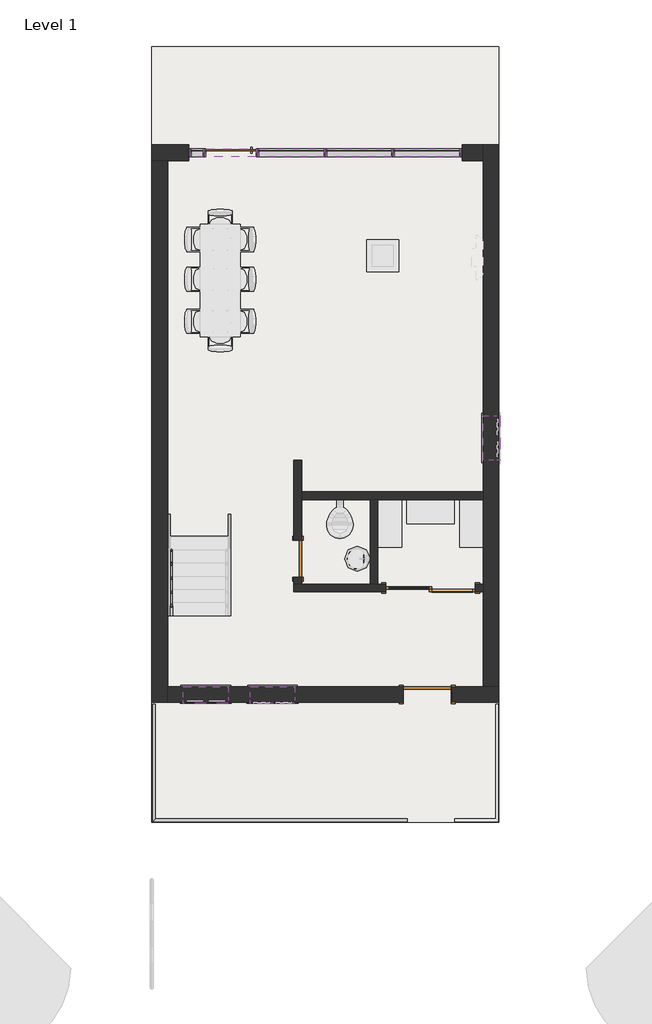
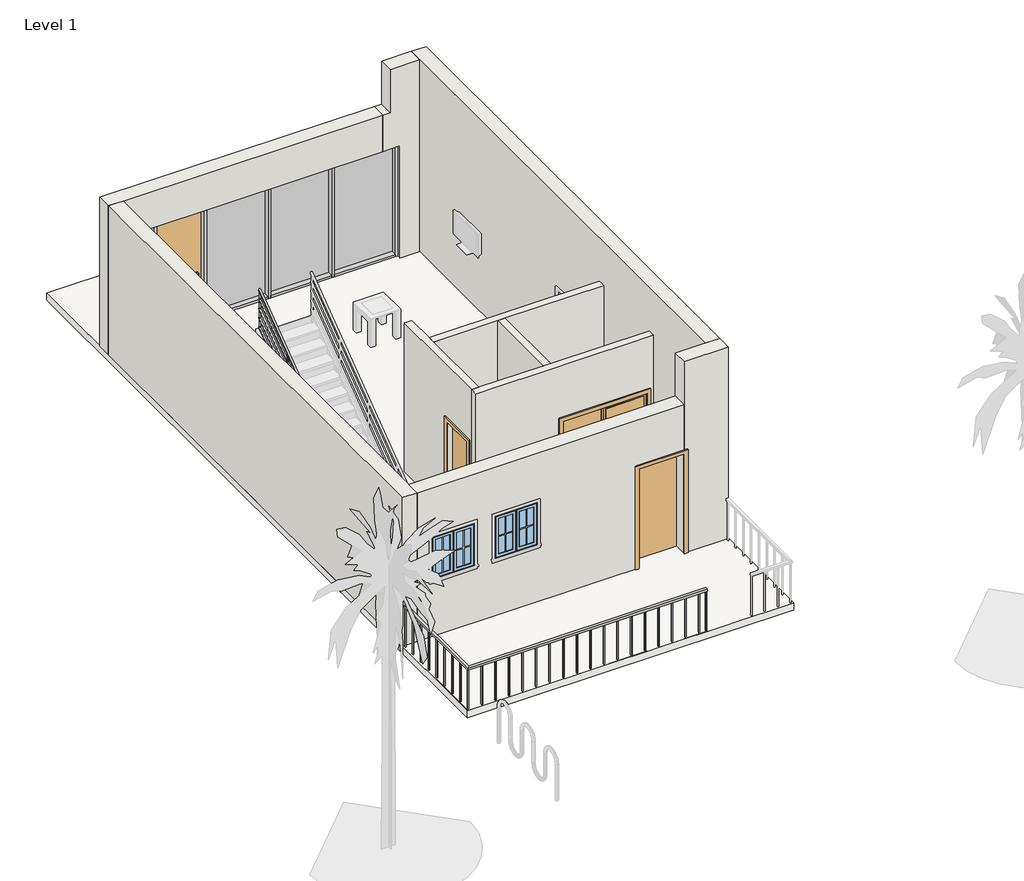
# One storey, part 1 of 2: 15 members, 10 walls, 4 doors, 4 plates, 3 windows, 2 railings, 1 slab.
"""IFC4 building model written with IfcOpenShell, lengths in millimetres."""

from ifc_helpers import new_model, si_unit, frame, origin, origin_with_axes, place, context, project, spatial, polyline, circle_curve, ellipse_curve, outline, extrude, faceted_brep, transform, mapped, element, save
from ifc_brep_helpers import plane_surface, cylinder_surface, advanced_brep
from components import m_door_curtain_wall_single_glass_m_door_curtain_wall_single_92f462ab, m_door_double_sliding_1700_x_2000mm_d36f6dca, m_single_flush_0915_x_2134mm_9cebaac8, m_single_flush_700x1980_d4223ffa, rectangular_mullion_50_x_150mm_6225e4e3, rectangular_mullion_50_x_150mm_662c37b1, rectangular_mullion_50_x_150mm_ef1c4831, rectangular_mullion_50_x_150mm_c6e312d8, rectangular_mullion_50_x_150mm_a74c1b10, rectangular_mullion_50_x_150mm_bd48bb75, system_panel_glazed_6a0df73a, system_panel_glazed_b955046d, m_window_casement_double_850_x_900mm_d87c3818, m_window_casement_double_850_x_900mm_ced1a82e

model = new_model("IFC4")

# Units and contexts
model_context = context("Model", 3, world=origin())
ifc_project = project(units=[si_unit("LENGTHUNIT", "METRE", prefix="MILLI")], contexts=[model_context])

# Site, building, storey
site = spatial("IfcSite", under=ifc_project)
building = spatial("IfcBuilding", under=site)
storey = spatial("IfcBuildingStorey", under=building, Name="Level 1", Elevation=0.0)

# Doors
placement = place(None, origin())
m_door_curtain_wall_single_glass_m_door_curtain_wall_single_shape = m_door_curtain_wall_single_glass_m_door_curtain_wall_single_92f462ab(model_context)
element("IfcDoor", 1, ObjectType="M_Door-Curtain-Wall-Single-Glass : M_Door-Curtain-Wall-Single-Glass", at=placement, inside=storey, context=model_context, shape_type="MappedRepresentation", body=[
    mapped(m_door_curtain_wall_single_glass_m_door_curtain_wall_single_shape, transform((-3862.7817551, 6033.2522499, 0.0), x_axis=(-1.0, 0.0, 0.0), y_axis=(0.0, -1.0, 0.0), z_axis=(0.0, 0.0, 1.0))),
])
m_door_double_sliding_1700_x_2000mm_shape = m_door_double_sliding_1700_x_2000mm_d36f6dca(model_context)
element("IfcDoor", 2, ObjectType="M_Door-Double-Sliding : 1700 x 2000mm", at=placement, inside=storey, context=model_context, shape_type="MappedRepresentation", body=[
    mapped(m_door_double_sliding_1700_x_2000mm_shape, transform((-69.0317552, -2114.7477501, 0.0), x_axis=(-1.0, 0.0, 0.0), y_axis=(0.0, -1.0, 0.0), z_axis=(0.0, 0.0, 1.0))),
])
m_single_flush_0915_x_2134mm_shape = m_single_flush_0915_x_2134mm_9cebaac8(model_context)
element("IfcDoor", 3, ObjectType="M_Single-Flush : 0915 x 2134mm", at=placement, inside=storey, context=model_context, shape_type="MappedRepresentation", body=[
    mapped(m_single_flush_0915_x_2134mm_shape, transform((-131.5317552, -4266.7477501, 0.0), x_axis=(1.0, 0.0, 0.0), y_axis=(0.0, 1.0, 0.0), z_axis=(0.0, 0.0, 1.0))),
])
m_single_flush_700x1980_shape = m_single_flush_700x1980_d4223ffa(model_context)
element("IfcDoor", 4, ObjectType="M_Single-Flush : 700x1980", at=placement, inside=storey, context=model_context, shape_type="MappedRepresentation", body=[
    mapped(m_single_flush_700x1980_shape, transform((-2594.0317552, -1685.7477501, 0.0), x_axis=(0.0, -1.0, 0.0), y_axis=(1.0, 0.0, 0.0), z_axis=(0.0, 0.0, 1.0))),
])

# Members
rectangular_mullion_50_x_150mm_shape = rectangular_mullion_50_x_150mm_6225e4e3(model_context)
element("IfcMember", 5, ObjectType="Rectangular Mullion : 50 x 150mm", at=placement, inside=storey, context=model_context, shape_type="MappedRepresentation", body=[
    mapped(rectangular_mullion_50_x_150mm_shape, transform((-3356.531755, 6033.2522499, 0.0), x_axis=(1.0, 0.0, 0.0), y_axis=(0.0, -1.0, 0.0), z_axis=(0.0, 0.0, -1.0))),
])
element("IfcMember", 6, ObjectType="Rectangular Mullion : 50 x 150mm", at=placement, inside=storey, context=model_context, shape_type="MappedRepresentation", body=[
    mapped(rectangular_mullion_50_x_150mm_shape, transform((-2069.0317552, 6033.2522499, 0.0), x_axis=(1.0, 0.0, 0.0), y_axis=(0.0, -1.0, 0.0), z_axis=(0.0, 0.0, -1.0))),
])
element("IfcMember", 7, ObjectType="Rectangular Mullion : 50 x 150mm", at=placement, inside=storey, context=model_context, shape_type="MappedRepresentation", body=[
    mapped(rectangular_mullion_50_x_150mm_shape, transform((-781.5317553, 6033.2522499, 0.0), x_axis=(1.0, 0.0, 0.0), y_axis=(0.0, -1.0, 0.0), z_axis=(0.0, 0.0, -1.0))),
])
element("IfcMember", 8, ObjectType="Rectangular Mullion : 50 x 150mm", at=placement, inside=storey, context=model_context, shape_type="MappedRepresentation", body=[
    mapped(rectangular_mullion_50_x_150mm_shape, transform((-4369.0317552, 6033.2522499, 0.0), x_axis=(1.0, 0.0, 0.0), y_axis=(0.0, -1.0, 0.0), z_axis=(0.0, 0.0, -1.0))),
])
rectangular_mullion_50_x_150mm_2_shape = rectangular_mullion_50_x_150mm_662c37b1(model_context)
element("IfcMember", 9, ObjectType="Rectangular Mullion : 50 x 150mm", at=placement, inside=storey, context=model_context, shape_type="MappedRepresentation", body=[
    mapped(rectangular_mullion_50_x_150mm_2_shape, transform((530.9682448, 6033.2522499, 0.0), x_axis=(1.0, 0.0, 0.0), y_axis=(0.0, -1.0, 0.0), z_axis=(0.0, 0.0, -1.0))),
])
element("IfcMember", 10, ObjectType="Rectangular Mullion : 50 x 150mm", at=placement, inside=storey, context=model_context, shape_type="MappedRepresentation", body=[
    mapped(rectangular_mullion_50_x_150mm_2_shape, transform((-4669.0317552, 6033.2522499, 2400.0), x_axis=(-1.0, 0.0, 0.0), y_axis=(0.0, -1.0, 0.0), z_axis=(0.0, 0.0, 1.0))),
])
rectangular_mullion_50_x_150mm_3_shape = rectangular_mullion_50_x_150mm_ef1c4831(model_context)
element("IfcMember", 11, ObjectType="Rectangular Mullion : 50 x 150mm", at=placement, inside=storey, context=model_context, shape_type="MappedRepresentation", body=[
    mapped(rectangular_mullion_50_x_150mm_3_shape, transform((-4619.0317552, 6033.2522499, 0.0), x_axis=(0.0, 0.0, -1.0), y_axis=(0.0, -1.0, 0.0), z_axis=(-1.0, 0.0, 0.0))),
])
element("IfcMember", 12, ObjectType="Rectangular Mullion : 50 x 150mm", at=placement, inside=storey, context=model_context, shape_type="MappedRepresentation", body=[
    mapped(rectangular_mullion_50_x_150mm_3_shape, transform((-4394.0317552, 6033.2522499, 2400.0), x_axis=(0.0, 0.0, 1.0), y_axis=(0.0, -1.0, 0.0), z_axis=(1.0, 0.0, 0.0))),
])
rectangular_mullion_50_x_150mm_4_shape = rectangular_mullion_50_x_150mm_c6e312d8(model_context)
element("IfcMember", 13, ObjectType="Rectangular Mullion : 50 x 150mm", at=placement, inside=storey, context=model_context, shape_type="MappedRepresentation", body=[
    mapped(rectangular_mullion_50_x_150mm_4_shape, transform((480.9682448, 6033.2522499, 2400.0), x_axis=(0.0, 0.0, 1.0), y_axis=(0.0, -1.0, 0.0), z_axis=(1.0, 0.0, 0.0))),
])
element("IfcMember", 14, ObjectType="Rectangular Mullion : 50 x 150mm", at=placement, inside=storey, context=model_context, shape_type="MappedRepresentation", body=[
    mapped(rectangular_mullion_50_x_150mm_4_shape, transform((-2094.0317552, 6033.2522499, 2400.0), x_axis=(0.0, 0.0, 1.0), y_axis=(0.0, -1.0, 0.0), z_axis=(1.0, 0.0, 0.0))),
])
element("IfcMember", 15, ObjectType="Rectangular Mullion : 50 x 150mm", at=placement, inside=storey, context=model_context, shape_type="MappedRepresentation", body=[
    mapped(rectangular_mullion_50_x_150mm_4_shape, transform((-806.5317553, 6033.2522499, 2400.0), x_axis=(0.0, 0.0, 1.0), y_axis=(0.0, -1.0, 0.0), z_axis=(1.0, 0.0, 0.0))),
])
rectangular_mullion_50_x_150mm_5_shape = rectangular_mullion_50_x_150mm_a74c1b10(model_context)
element("IfcMember", 16, ObjectType="Rectangular Mullion : 50 x 150mm", at=placement, inside=storey, context=model_context, shape_type="MappedRepresentation", body=[
    mapped(rectangular_mullion_50_x_150mm_5_shape, transform((-3381.531755, 6033.2522499, 2400.0), x_axis=(0.0, 0.0, 1.0), y_axis=(0.0, -1.0, 0.0), z_axis=(1.0, 0.0, 0.0))),
])
rectangular_mullion_50_x_150mm_6_shape = rectangular_mullion_50_x_150mm_bd48bb75(model_context)
element("IfcMember", 17, ObjectType="Rectangular Mullion : 50 x 150mm", at=placement, inside=storey, context=model_context, shape_type="MappedRepresentation", body=[
    mapped(rectangular_mullion_50_x_150mm_6_shape, transform((-3331.531755, 6033.2522499, 0.0), x_axis=(0.0, 0.0, -1.0), y_axis=(0.0, -1.0, 0.0), z_axis=(-1.0, 0.0, 0.0))),
])
element("IfcMember", 18, ObjectType="Rectangular Mullion : 50 x 150mm", at=placement, inside=storey, context=model_context, shape_type="MappedRepresentation", body=[
    mapped(rectangular_mullion_50_x_150mm_6_shape, transform((-2044.0317552, 6033.2522499, 0.0), x_axis=(0.0, 0.0, -1.0), y_axis=(0.0, -1.0, 0.0), z_axis=(-1.0, 0.0, 0.0))),
])
element("IfcMember", 19, ObjectType="Rectangular Mullion : 50 x 150mm", at=placement, inside=storey, context=model_context, shape_type="MappedRepresentation", body=[
    mapped(rectangular_mullion_50_x_150mm_6_shape, transform((-756.5317553, 6033.2522499, 0.0), x_axis=(0.0, 0.0, -1.0), y_axis=(0.0, -1.0, 0.0), z_axis=(-1.0, 0.0, 0.0))),
])

# Plates
system_panel_glazed_shape = system_panel_glazed_6a0df73a(model_context)
element("IfcPlate", 20, ObjectType="System Panel : Glazed", at=placement, inside=storey, context=model_context, shape_type="MappedRepresentation", body=[
    mapped(system_panel_glazed_shape, transform((-4506.5317552, 6033.2522499, 50.0), x_axis=(1.0, 0.0, 0.0), y_axis=(0.0, 1.0, 0.0), z_axis=(0.0, 0.0, 1.0))),
])
system_panel_glazed_2_shape = system_panel_glazed_b955046d(model_context)
element("IfcPlate", 21, ObjectType="System Panel : Glazed", at=placement, inside=storey, context=model_context, shape_type="MappedRepresentation", body=[
    mapped(system_panel_glazed_2_shape, transform((-137.7817553, 6033.2522499, 50.0), x_axis=(1.0, 0.0, 0.0), y_axis=(0.0, 1.0, 0.0), z_axis=(0.0, 0.0, 1.0))),
])
element("IfcPlate", 22, ObjectType="System Panel : Glazed", at=placement, inside=storey, context=model_context, shape_type="MappedRepresentation", body=[
    mapped(system_panel_glazed_2_shape, transform((-1425.2817553, 6033.2522499, 50.0), x_axis=(1.0, 0.0, 0.0), y_axis=(0.0, 1.0, 0.0), z_axis=(0.0, 0.0, 1.0))),
])
element("IfcPlate", 23, ObjectType="System Panel : Glazed", at=placement, inside=storey, context=model_context, shape_type="MappedRepresentation", body=[
    mapped(system_panel_glazed_2_shape, transform((-2712.7817551, 6033.2522499, 50.0), x_axis=(1.0, 0.0, 0.0), y_axis=(0.0, 1.0, 0.0), z_axis=(0.0, 0.0, 1.0))),
])

# Railings
element("IfcRailing", 24, ObjectType="900mm Pipe", at=placement, inside=storey, context=model_context, shape_type="AdvancedBrep", body=[
    advanced_brep(
    [(-4973.6317552, -2766.7477501, 1063.1999558), (-5013.6317552, -2766.7477501, 1063.1999558), (-4973.6317552, 1233.2522499, 4074.9646617), (-5013.6317552, 1233.2522499, 4074.9646617)],
    [
        (0, 1, ellipse_curve(frame((-4993.6317552, -2766.7477501, 1063.1999558), z_axis=(0.0, -1.0, 0.0), x_axis=(0.0, 0.0, -1.0)), 25.0353383, 20.0)),
        (1, 0, ellipse_curve(frame((-4993.6317552, -2766.7477501, 1063.1999558), z_axis=(0.0, -1.0, 0.0), x_axis=(0.0, 0.0, -1.0)), 25.0353383, 20.0)),
        (2, 3, ellipse_curve(frame((-4993.6317552, 1233.2522499, 4074.9646617), z_axis=(0.0, 1.0, 0.0), x_axis=(0.0, 0.0, -1.0)), 25.0353383, 20.0)),
        (3, 2, ellipse_curve(frame((-4993.6317552, 1233.2522499, 4074.9646617), z_axis=(0.0, 1.0, 0.0), x_axis=(0.0, 0.0, -1.0)), 25.0353383, 20.0)),
        (0, 2),
        (3, 1),
    ],
    [
        plane_surface(frame((-4993.6317552, -2766.7477501, 1088.2352941), z_axis=(0.0, -1.0, 0.0), x_axis=(0.0, 0.0, 1.0))),
        plane_surface(frame((-4993.6317552, 1233.2522499, 4100.0), z_axis=(0.0, 1.0, 0.0), x_axis=(0.0, 0.0, 1.0))),
        cylinder_surface(frame((-4993.6317552, -2754.7176962, 1072.2578787), z_axis=(0.0, -0.7988707691396074, -0.6015026967639399), x_axis=(-1.0, 0.0, 0.0)), 20.0),
    ],
    [
        (0, [[1, 2]]),
        (1, [[3, 4]]),
        (2, [[-1, 5, -4, 6]]),
        (2, [[-2, -6, -3, -5]]),
    ],
),
    advanced_brep(
    [(-4978.6317552, -2766.7477501, 869.4587904), (-5008.6317552, -2766.7477501, 869.4587904), (-4978.6317552, 1233.2522499, 3881.2234962), (-5008.6317552, 1233.2522499, 3881.2234962)],
    [
        (0, 1, ellipse_curve(frame((-4993.6317552, -2766.7477501, 869.4587904), z_axis=(0.0, -1.0, 0.0), x_axis=(0.0, 0.0, -1.0)), 18.7765038, 15.0)),
        (1, 0, ellipse_curve(frame((-4993.6317552, -2766.7477501, 869.4587904), z_axis=(0.0, -1.0, 0.0), x_axis=(0.0, 0.0, -1.0)), 18.7765038, 15.0)),
        (2, 3, ellipse_curve(frame((-4993.6317552, 1233.2522499, 3881.2234962), z_axis=(0.0, 1.0, 0.0), x_axis=(0.0, 0.0, -1.0)), 18.7765038, 15.0)),
        (3, 2, ellipse_curve(frame((-4993.6317552, 1233.2522499, 3881.2234962), z_axis=(0.0, 1.0, 0.0), x_axis=(0.0, 0.0, -1.0)), 18.7765038, 15.0)),
        (0, 2),
        (3, 1),
    ],
    [
        plane_surface(frame((-4993.6317552, -2766.7477501, 888.2352941), z_axis=(0.0, -1.0, 0.0), x_axis=(0.0, 0.0, 1.0))),
        plane_surface(frame((-4993.6317552, 1233.2522499, 3900.0), z_axis=(0.0, 1.0, 0.0), x_axis=(0.0, 0.0, 1.0))),
        cylinder_surface(frame((-4993.6317552, -2757.7252097, 876.2522326), z_axis=(0.0, -0.7988707691396074, -0.6015026967639399), x_axis=(-1.0, 0.0, 0.0)), 15.0),
    ],
    [
        (0, [[1, 2]]),
        (1, [[3, 4]]),
        (2, [[-1, 5, -4, 6]]),
        (2, [[-2, -6, -3, -5]]),
    ],
),
    advanced_brep(
    [(-4978.6317552, -2766.7477501, 669.4587904), (-5008.6317552, -2766.7477501, 669.4587904), (-4978.6317552, 1233.2522499, 3681.2234962), (-5008.6317552, 1233.2522499, 3681.2234962)],
    [
        (0, 1, ellipse_curve(frame((-4993.6317552, -2766.7477501, 669.4587904), z_axis=(0.0, -1.0, 0.0), x_axis=(0.0, 0.0, -1.0)), 18.7765038, 15.0)),
        (1, 0, ellipse_curve(frame((-4993.6317552, -2766.7477501, 669.4587904), z_axis=(0.0, -1.0, 0.0), x_axis=(0.0, 0.0, -1.0)), 18.7765038, 15.0)),
        (2, 3, ellipse_curve(frame((-4993.6317552, 1233.2522499, 3681.2234962), z_axis=(0.0, 1.0, 0.0), x_axis=(0.0, 0.0, -1.0)), 18.7765038, 15.0)),
        (3, 2, ellipse_curve(frame((-4993.6317552, 1233.2522499, 3681.2234962), z_axis=(0.0, 1.0, 0.0), x_axis=(0.0, 0.0, -1.0)), 18.7765038, 15.0)),
        (0, 2),
        (3, 1),
    ],
    [
        plane_surface(frame((-4993.6317552, -2766.7477501, 688.2352941), z_axis=(0.0, -1.0, 0.0), x_axis=(0.0, 0.0, 1.0))),
        plane_surface(frame((-4993.6317552, 1233.2522499, 3700.0), z_axis=(0.0, 1.0, 0.0), x_axis=(0.0, 0.0, 1.0))),
        cylinder_surface(frame((-4993.6317552, -2757.7252097, 676.2522326), z_axis=(0.0, -0.7988707691396074, -0.6015026967639399), x_axis=(-1.0, 0.0, 0.0)), 15.0),
    ],
    [
        (0, [[1, 2]]),
        (1, [[3, 4]]),
        (2, [[-1, 5, -4, 6]]),
        (2, [[-2, -6, -3, -5]]),
    ],
),
    advanced_brep(
    [(-4978.6317552, -2766.7477501, 469.4587904), (-5008.6317552, -2766.7477501, 469.4587904), (-4978.6317552, 1233.2522499, 3481.2234962), (-5008.6317552, 1233.2522499, 3481.2234962)],
    [
        (0, 1, ellipse_curve(frame((-4993.6317552, -2766.7477501, 469.4587904), z_axis=(0.0, -1.0, 0.0), x_axis=(0.0, 0.0, -1.0)), 18.7765038, 15.0)),
        (1, 0, ellipse_curve(frame((-4993.6317552, -2766.7477501, 469.4587904), z_axis=(0.0, -1.0, 0.0), x_axis=(0.0, 0.0, -1.0)), 18.7765038, 15.0)),
        (2, 3, ellipse_curve(frame((-4993.6317552, 1233.2522499, 3481.2234962), z_axis=(0.0, 1.0, 0.0), x_axis=(0.0, 0.0, -1.0)), 18.7765038, 15.0)),
        (3, 2, ellipse_curve(frame((-4993.6317552, 1233.2522499, 3481.2234962), z_axis=(0.0, 1.0, 0.0), x_axis=(0.0, 0.0, -1.0)), 18.7765038, 15.0)),
        (0, 2),
        (3, 1),
    ],
    [
        plane_surface(frame((-4993.6317552, -2766.7477501, 488.2352941), z_axis=(0.0, -1.0, 0.0), x_axis=(0.0, 0.0, 1.0))),
        plane_surface(frame((-4993.6317552, 1233.2522499, 3500.0), z_axis=(0.0, 1.0, 0.0), x_axis=(0.0, 0.0, 1.0))),
        cylinder_surface(frame((-4993.6317552, -2757.7252097, 476.2522326), z_axis=(0.0, -0.7988707691396074, -0.6015026967639399), x_axis=(-1.0, 0.0, 0.0)), 15.0),
    ],
    [
        (0, [[1, 2]]),
        (1, [[3, 4]]),
        (2, [[-1, 5, -4, 6]]),
        (2, [[-2, -6, -3, -5]]),
    ],
),
    advanced_brep(
    [(-4978.6317552, -2766.7477501, 269.4587904), (-5008.6317552, -2766.7477501, 269.4587904), (-4978.6317552, 1233.2522499, 3281.2234962), (-5008.6317552, 1233.2522499, 3281.2234962)],
    [
        (0, 1, ellipse_curve(frame((-4993.6317552, -2766.7477501, 269.4587904), z_axis=(0.0, -1.0, 0.0), x_axis=(0.0, 0.0, -1.0)), 18.7765038, 15.0)),
        (1, 0, ellipse_curve(frame((-4993.6317552, -2766.7477501, 269.4587904), z_axis=(0.0, -1.0, 0.0), x_axis=(0.0, 0.0, -1.0)), 18.7765038, 15.0)),
        (2, 3, ellipse_curve(frame((-4993.6317552, 1233.2522499, 3281.2234962), z_axis=(0.0, 1.0, 0.0), x_axis=(0.0, 0.0, -1.0)), 18.7765038, 15.0)),
        (3, 2, ellipse_curve(frame((-4993.6317552, 1233.2522499, 3281.2234962), z_axis=(0.0, 1.0, 0.0), x_axis=(0.0, 0.0, -1.0)), 18.7765038, 15.0)),
        (0, 2),
        (3, 1),
    ],
    [
        plane_surface(frame((-4993.6317552, -2766.7477501, 288.2352941), z_axis=(0.0, -1.0, 0.0), x_axis=(0.0, 0.0, 1.0))),
        plane_surface(frame((-4993.6317552, 1233.2522499, 3300.0), z_axis=(0.0, 1.0, 0.0), x_axis=(0.0, 0.0, 1.0))),
        cylinder_surface(frame((-4993.6317552, -2757.7252097, 276.2522326), z_axis=(0.0, -0.7988707691396074, -0.6015026967639399), x_axis=(-1.0, 0.0, 0.0)), 15.0),
    ],
    [
        (0, [[1, 2]]),
        (1, [[3, 4]]),
        (2, [[-1, 5, -4, 6]]),
        (2, [[-2, -6, -3, -5]]),
    ],
),
    advanced_brep(
    [(-5006.1317552, 233.2522499, 3296.9881468), (-4981.1317552, 233.2522499, 3296.9881468), (-4981.1317552, 233.2522499, 2447.0588235), (-5006.1317552, 233.2522499, 2447.0588235)],
    [
        (0, 1, ellipse_curve(frame((-4993.6317552, 233.2522499, 3296.9881468), z_axis=(0.0, 0.6015026967639397, -0.7988707691396074), x_axis=(0.0, 0.7988707691396075, 0.6015026967639399)), 15.6470865, 12.5)),
        (1, 2),
        (2, 3, circle_curve(frame((-4993.6317552, 233.2522499, 2447.0588235), z_axis=(0.0, 0.0, 1.0), x_axis=(1.0, 0.0, 0.0)), 12.5)),
        (3, 0),
        (3, 2, circle_curve(frame((-4993.6317552, 233.2522499, 2447.0588235), z_axis=(0.0, 0.0, 1.0), x_axis=(1.0, 0.0, 0.0)), 12.5)),
        (1, 0, ellipse_curve(frame((-4993.6317552, 233.2522499, 3296.9881468), z_axis=(0.0, 0.6015026967639397, -0.7988707691396074), x_axis=(0.0, 0.7988707691396075, 0.6015026967639399)), 15.6470865, 12.5)),
    ],
    [
        cylinder_surface(frame((-4993.6317552, 233.2522499, 2347.0588235), z_axis=(0.0, 0.0, 1.0), x_axis=(1.0, 0.0, 0.0)), 12.5),
        plane_surface(frame((-4968.6317552, 258.2522499, 3315.8116762), z_axis=(0.0, -0.6015026967639397, 0.7988707691396074), x_axis=(-1.0, 0.0, 0.0))),
        plane_surface(frame((-4968.6317552, 208.2522499, 2447.0588235), z_axis=(0.0, 0.0, -1.0), x_axis=(-1.0, 0.0, 0.0))),
    ],
    [
        (0, [[1, 2, 3, 4]]),
        (0, [[5, -2, 6, -4]]),
        (1, [[-6, -1]]),
        (2, [[-5, -3]]),
    ],
),
    advanced_brep(
    [(-5006.1317552, -766.7477501, 2544.0469704), (-4981.1317552, -766.7477501, 2544.0469704), (-4981.1317552, -766.7477501, 1694.1176471), (-5006.1317552, -766.7477501, 1694.1176471)],
    [
        (0, 1, ellipse_curve(frame((-4993.6317552, -766.7477501, 2544.0469704), z_axis=(0.0, 0.6015026967639397, -0.7988707691396074), x_axis=(0.0, 0.7988707691396075, 0.6015026967639399)), 15.6470865, 12.5)),
        (1, 2),
        (2, 3, circle_curve(frame((-4993.6317552, -766.7477501, 1694.1176471), z_axis=(0.0, 0.0, 1.0), x_axis=(1.0, 0.0, 0.0)), 12.5)),
        (3, 0),
        (3, 2, circle_curve(frame((-4993.6317552, -766.7477501, 1694.1176471), z_axis=(0.0, 0.0, 1.0), x_axis=(1.0, 0.0, 0.0)), 12.5)),
        (1, 0, ellipse_curve(frame((-4993.6317552, -766.7477501, 2544.0469704), z_axis=(0.0, 0.6015026967639397, -0.7988707691396074), x_axis=(0.0, 0.7988707691396075, 0.6015026967639399)), 15.6470865, 12.5)),
    ],
    [
        cylinder_surface(frame((-4993.6317552, -766.7477501, 1594.1176471), z_axis=(0.0, 0.0, 1.0), x_axis=(1.0, 0.0, 0.0)), 12.5),
        plane_surface(frame((-4968.6317552, -741.7477501, 2562.8704998), z_axis=(0.0, -0.6015026967639397, 0.7988707691396074), x_axis=(-1.0, 0.0, 0.0))),
        plane_surface(frame((-4968.6317552, -791.7477501, 1694.1176471), z_axis=(0.0, 0.0, -1.0), x_axis=(-1.0, 0.0, 0.0))),
    ],
    [
        (0, [[1, 2, 3, 4]]),
        (0, [[5, -2, 6, -4]]),
        (1, [[-6, -1]]),
        (2, [[-5, -3]]),
    ],
),
    advanced_brep(
    [(-5006.1317552, -1766.7477501, 1791.1057939), (-4981.1317552, -1766.7477501, 1791.1057939), (-4981.1317552, -1766.7477501, 941.1764706), (-5006.1317552, -1766.7477501, 941.1764706)],
    [
        (0, 1, ellipse_curve(frame((-4993.6317552, -1766.7477501, 1791.1057939), z_axis=(0.0, 0.6015026967639397, -0.7988707691396074), x_axis=(0.0, 0.7988707691396075, 0.6015026967639399)), 15.6470865, 12.5)),
        (1, 2),
        (2, 3, circle_curve(frame((-4993.6317552, -1766.7477501, 941.1764706), z_axis=(0.0, 0.0, 1.0), x_axis=(1.0, 0.0, 0.0)), 12.5)),
        (3, 0),
        (3, 2, circle_curve(frame((-4993.6317552, -1766.7477501, 941.1764706), z_axis=(0.0, 0.0, 1.0), x_axis=(1.0, 0.0, 0.0)), 12.5)),
        (1, 0, ellipse_curve(frame((-4993.6317552, -1766.7477501, 1791.1057939), z_axis=(0.0, 0.6015026967639397, -0.7988707691396074), x_axis=(0.0, 0.7988707691396075, 0.6015026967639399)), 15.6470865, 12.5)),
    ],
    [
        cylinder_surface(frame((-4993.6317552, -1766.7477501, 841.1764706), z_axis=(0.0, 0.0, 1.0), x_axis=(1.0, 0.0, 0.0)), 12.5),
        plane_surface(frame((-4968.6317552, -1741.7477501, 1809.9293233), z_axis=(0.0, -0.6015026967639397, 0.7988707691396074), x_axis=(-1.0, 0.0, 0.0))),
        plane_surface(frame((-4968.6317552, -1791.7477501, 941.1764706), z_axis=(0.0, 0.0, -1.0), x_axis=(-1.0, 0.0, 0.0))),
    ],
    [
        (0, [[1, 2, 3, 4]]),
        (0, [[5, -2, 6, -4]]),
        (1, [[-6, -1]]),
        (2, [[-5, -3]]),
    ],
),
    advanced_brep(
    [(-5006.1317552, 1220.7522499, 4040.5175586), (-4981.1317552, 1220.7522499, 4040.5175586), (-4981.1317552, 1220.7522499, 3011.7647059), (-5006.1317552, 1220.7522499, 3011.7647059)],
    [
        (0, 1, ellipse_curve(frame((-4993.6317552, 1220.7522499, 4040.5175586), z_axis=(0.0, 0.6015026967639397, -0.7988707691396074), x_axis=(0.0, 0.7988707691396075, 0.6015026967639399)), 15.6470865, 12.5)),
        (1, 2),
        (2, 3, circle_curve(frame((-4993.6317552, 1220.7522499, 3011.7647059), z_axis=(0.0, 0.0, 1.0), x_axis=(1.0, 0.0, 0.0)), 12.5)),
        (3, 0),
        (3, 2, circle_curve(frame((-4993.6317552, 1220.7522499, 3011.7647059), z_axis=(0.0, 0.0, 1.0), x_axis=(1.0, 0.0, 0.0)), 12.5)),
        (1, 0, ellipse_curve(frame((-4993.6317552, 1220.7522499, 4040.5175586), z_axis=(0.0, 0.6015026967639397, -0.7988707691396074), x_axis=(0.0, 0.7988707691396075, 0.6015026967639399)), 15.6470865, 12.5)),
    ],
    [
        cylinder_surface(frame((-4993.6317552, 1220.7522499, 2911.7647059), z_axis=(0.0, 0.0, 1.0), x_axis=(1.0, 0.0, 0.0)), 12.5),
        plane_surface(frame((-4968.6317552, 1245.7522499, 4059.341088), z_axis=(0.0, -0.6015026967639397, 0.7988707691396074), x_axis=(-1.0, 0.0, 0.0))),
        plane_surface(frame((-4968.6317552, 1195.7522499, 3011.7647059), z_axis=(0.0, 0.0, -1.0), x_axis=(-1.0, 0.0, 0.0))),
    ],
    [
        (0, [[1, 2, 3, 4]]),
        (0, [[5, -2, 6, -4]]),
        (1, [[-6, -1]]),
        (2, [[-5, -3]]),
    ],
),
    advanced_brep(
    [(-5006.1317552, -2754.2477501, 1047.5763821), (-4981.1317552, -2754.2477501, 1047.5763821), (-4981.1317552, -2754.2477501, 188.2352941), (-5006.1317552, -2754.2477501, 188.2352941)],
    [
        (0, 1, ellipse_curve(frame((-4993.6317552, -2754.2477501, 1047.5763821), z_axis=(0.0, 0.6015026967639397, -0.7988707691396074), x_axis=(0.0, 0.7988707691396075, 0.6015026967639399)), 15.6470865, 12.5)),
        (1, 2),
        (2, 3, circle_curve(frame((-4993.6317552, -2754.2477501, 188.2352941), z_axis=(0.0, 0.0, 1.0), x_axis=(1.0, 0.0, 0.0)), 12.5)),
        (3, 0),
        (3, 2, circle_curve(frame((-4993.6317552, -2754.2477501, 188.2352941), z_axis=(0.0, 0.0, 1.0), x_axis=(1.0, 0.0, 0.0)), 12.5)),
        (1, 0, ellipse_curve(frame((-4993.6317552, -2754.2477501, 1047.5763821), z_axis=(0.0, 0.6015026967639397, -0.7988707691396074), x_axis=(0.0, 0.7988707691396075, 0.6015026967639399)), 15.6470865, 12.5)),
    ],
    [
        cylinder_surface(frame((-4993.6317552, -2754.2477501, 88.2352941), z_axis=(0.0, 0.0, 1.0), x_axis=(1.0, 0.0, 0.0)), 12.5),
        plane_surface(frame((-4968.6317552, -2729.2477501, 1066.3999115), z_axis=(0.0, -0.6015026967639397, 0.7988707691396074), x_axis=(-1.0, 0.0, 0.0))),
        plane_surface(frame((-4968.6317552, -2779.2477501, 188.2352941), z_axis=(0.0, 0.0, -1.0), x_axis=(-1.0, 0.0, 0.0))),
    ],
    [
        (0, [[1, 2, 3, 4]]),
        (0, [[5, -2, 6, -4]]),
        (1, [[-6, -1]]),
        (2, [[-5, -3]]),
    ],
),
])
element("IfcRailing", 25, ObjectType="NEW RAILING", at=placement, inside=storey, context=model_context, shape_type="SolidModel", body=[
    faceted_brep([(-5304.0317552, -4455.3361723, 900.0), (-5304.0317552, -4455.3361723, 850.0), (-5354.0317552, -4455.3361723, 850.0), (-5354.0317552, -4455.3361723, 900.0), (-509.0317552, -6630.3361723, 900.0), (-509.0317552, -6680.3361723, 900.0), (-509.0317552, -6680.3361723, 850.0), (-509.0317552, -6630.3361723, 850.0), (-5304.0317552, -6630.3361723, 900.0), (-5304.0317552, -6630.3361723, 850.0), (-5354.0317552, -6680.3361723, 850.0), (-5354.0317552, -6680.3361723, 900.0)], [[[0, 1, 2, 3]], [[4, 5, 6, 7]], [[1, 0, 8, 9]], [[2, 1, 9, 10]], [[3, 2, 10, 11]], [[0, 3, 11, 8]], [[9, 8, 4, 7]], [[10, 9, 7, 6]], [[11, 10, 6, 5]], [[8, 11, 5, 4]]]),
    faceted_brep([(-5304.0317552, -4455.3361723, 0.0), (-5304.0317552, -4455.3361723, -60.0), (-5354.0317552, -4455.3361723, -60.0), (-5354.0317552, -4455.3361723, 0.0), (-5304.0317552, -6630.3361723, -60.0), (-5354.0317552, -6680.3361723, -60.0), (-5304.0317552, -6630.3361723, 0.0), (-509.0317552, -6630.3361723, 0.0), (-509.0317552, -6680.3361723, 0.0), (-509.0317552, -6680.3361723, -60.0), (-509.0317552, -6630.3361723, -60.0), (-5354.0317552, -6680.3361723, 0.0)], [[[0, 1, 2, 3]], [[2, 1, 4, 5]], [[1, 0, 6, 4]], [[7, 8, 9, 10]], [[5, 4, 10, 9]], [[4, 6, 7, 10]], [[3, 2, 5, 11]], [[0, 3, 11, 6]], [[11, 5, 9, 8]], [[6, 11, 8, 7]]]),
    extrude(outline(polyline([(-664.0317552, -6665.3361723), (-664.0317552, -6645.3361723), (-644.0317552, -6645.3361723), (-644.0317552, -6665.3361723), (-664.0317552, -6665.3361723)])), origin_with_axes(), (0.0, 0.0, 1.0), 850.0),
    extrude(outline(polyline([(-939.0317552, -6665.3361723), (-939.0317552, -6645.3361723), (-919.0317552, -6645.3361723), (-919.0317552, -6665.3361723), (-939.0317552, -6665.3361723)])), origin_with_axes(), (0.0, 0.0, 1.0), 850.0),
    extrude(outline(polyline([(-1214.0317552, -6665.3361723), (-1214.0317552, -6645.3361723), (-1194.0317552, -6645.3361723), (-1194.0317552, -6665.3361723), (-1214.0317552, -6665.3361723)])), origin_with_axes(), (0.0, 0.0, 1.0), 850.0),
    extrude(outline(polyline([(-1489.0317552, -6665.3361723), (-1489.0317552, -6645.3361723), (-1469.0317552, -6645.3361723), (-1469.0317552, -6665.3361723), (-1489.0317552, -6665.3361723)])), origin_with_axes(), (0.0, 0.0, 1.0), 850.0),
    extrude(outline(polyline([(-1764.0317552, -6665.3361723), (-1764.0317552, -6645.3361723), (-1744.0317552, -6645.3361723), (-1744.0317552, -6665.3361723), (-1764.0317552, -6665.3361723)])), origin_with_axes(), (0.0, 0.0, 1.0), 850.0),
    extrude(outline(polyline([(-2039.0317552, -6665.3361723), (-2039.0317552, -6645.3361723), (-2019.0317552, -6645.3361723), (-2019.0317552, -6665.3361723), (-2039.0317552, -6665.3361723)])), origin_with_axes(), (0.0, 0.0, 1.0), 850.0),
    extrude(outline(polyline([(-2314.0317552, -6665.3361723), (-2314.0317552, -6645.3361723), (-2294.0317552, -6645.3361723), (-2294.0317552, -6665.3361723), (-2314.0317552, -6665.3361723)])), origin_with_axes(), (0.0, 0.0, 1.0), 850.0),
    extrude(outline(polyline([(-2589.0317552, -6665.3361723), (-2589.0317552, -6645.3361723), (-2569.0317552, -6645.3361723), (-2569.0317552, -6665.3361723), (-2589.0317552, -6665.3361723)])), origin_with_axes(), (0.0, 0.0, 1.0), 850.0),
    extrude(outline(polyline([(-2864.0317552, -6665.3361723), (-2864.0317552, -6645.3361723), (-2844.0317552, -6645.3361723), (-2844.0317552, -6665.3361723), (-2864.0317552, -6665.3361723)])), origin_with_axes(), (0.0, 0.0, 1.0), 850.0),
    extrude(outline(polyline([(-3139.0317552, -6665.3361723), (-3139.0317552, -6645.3361723), (-3119.0317552, -6645.3361723), (-3119.0317552, -6665.3361723), (-3139.0317552, -6665.3361723)])), origin_with_axes(), (0.0, 0.0, 1.0), 850.0),
    extrude(outline(polyline([(-3414.0317552, -6665.3361723), (-3414.0317552, -6645.3361723), (-3394.0317552, -6645.3361723), (-3394.0317552, -6665.3361723), (-3414.0317552, -6665.3361723)])), origin_with_axes(), (0.0, 0.0, 1.0), 850.0),
    extrude(outline(polyline([(-3689.0317552, -6665.3361723), (-3689.0317552, -6645.3361723), (-3669.0317552, -6645.3361723), (-3669.0317552, -6665.3361723), (-3689.0317552, -6665.3361723)])), origin_with_axes(), (0.0, 0.0, 1.0), 850.0),
    extrude(outline(polyline([(-3964.0317552, -6665.3361723), (-3964.0317552, -6645.3361723), (-3944.0317552, -6645.3361723), (-3944.0317552, -6665.3361723), (-3964.0317552, -6665.3361723)])), origin_with_axes(), (0.0, 0.0, 1.0), 850.0),
    extrude(outline(polyline([(-4239.0317552, -6665.3361723), (-4239.0317552, -6645.3361723), (-4219.0317552, -6645.3361723), (-4219.0317552, -6665.3361723), (-4239.0317552, -6665.3361723)])), origin_with_axes(), (0.0, 0.0, 1.0), 850.0),
    extrude(outline(polyline([(-4514.0317552, -6665.3361723), (-4514.0317552, -6645.3361723), (-4494.0317552, -6645.3361723), (-4494.0317552, -6665.3361723), (-4514.0317552, -6665.3361723)])), origin_with_axes(), (0.0, 0.0, 1.0), 850.0),
    extrude(outline(polyline([(-4789.0317552, -6665.3361723), (-4789.0317552, -6645.3361723), (-4769.0317552, -6645.3361723), (-4769.0317552, -6665.3361723), (-4789.0317552, -6665.3361723)])), origin_with_axes(), (0.0, 0.0, 1.0), 850.0),
    extrude(outline(polyline([(-5064.0317552, -6665.3361723), (-5064.0317552, -6645.3361723), (-5044.0317552, -6645.3361723), (-5044.0317552, -6665.3361723), (-5064.0317552, -6665.3361723)])), origin_with_axes(), (0.0, 0.0, 1.0), 850.0),
    extrude(outline(polyline([(-5339.0317552, -6370.3361723), (-5319.0317552, -6370.3361723), (-5319.0317552, -6390.3361723), (-5339.0317552, -6390.3361723), (-5339.0317552, -6370.3361723)])), origin_with_axes(), (0.0, 0.0, 1.0), 850.0),
    extrude(outline(polyline([(-5339.0317552, -6095.3361723), (-5319.0317552, -6095.3361723), (-5319.0317552, -6115.3361723), (-5339.0317552, -6115.3361723), (-5339.0317552, -6095.3361723)])), origin_with_axes(), (0.0, 0.0, 1.0), 850.0),
    extrude(outline(polyline([(-5339.0317552, -5820.3361723), (-5319.0317552, -5820.3361723), (-5319.0317552, -5840.3361723), (-5339.0317552, -5840.3361723), (-5339.0317552, -5820.3361723)])), origin_with_axes(), (0.0, 0.0, 1.0), 850.0),
    extrude(outline(polyline([(-5339.0317552, -5545.3361723), (-5319.0317552, -5545.3361723), (-5319.0317552, -5565.3361723), (-5339.0317552, -5565.3361723), (-5339.0317552, -5545.3361723)])), origin_with_axes(), (0.0, 0.0, 1.0), 850.0),
    extrude(outline(polyline([(-5339.0317552, -5270.3361723), (-5319.0317552, -5270.3361723), (-5319.0317552, -5290.3361723), (-5339.0317552, -5290.3361723), (-5339.0317552, -5270.3361723)])), origin_with_axes(), (0.0, 0.0, 1.0), 850.0),
    extrude(outline(polyline([(-5339.0317552, -4995.3361723), (-5319.0317552, -4995.3361723), (-5319.0317552, -5015.3361723), (-5339.0317552, -5015.3361723), (-5339.0317552, -4995.3361723)])), origin_with_axes(), (0.0, 0.0, 1.0), 850.0),
    extrude(outline(polyline([(-5339.0317552, -4720.3361723), (-5319.0317552, -4720.3361723), (-5319.0317552, -4740.3361723), (-5339.0317552, -4740.3361723), (-5339.0317552, -4720.3361723)])), origin_with_axes(), (0.0, 0.0, 1.0), 850.0),
    extrude(outline(polyline([(-5339.0317552, -6645.3361723), (-5319.0317552, -6645.3361723), (-5319.0317552, -6665.3361723), (-5339.0317552, -6665.3361723), (-5339.0317552, -6645.3361723)])), origin_with_axes(), (0.0, 0.0, 1.0), 850.0),
    extrude(outline(polyline([(-529.0317552, -6665.3361723), (-529.0317552, -6645.3361723), (-509.0317552, -6645.3361723), (-509.0317552, -6665.3361723), (-529.0317552, -6665.3361723)])), origin_with_axes(), (0.0, 0.0, 1.0), 850.0),
    extrude(outline(polyline([(-5339.0317552, -4455.3361723), (-5319.0317552, -4455.3361723), (-5319.0317552, -4475.3361723), (-5339.0317552, -4475.3361723), (-5339.0317552, -4455.3361723)])), origin_with_axes(), (0.0, 0.0, 1.0), 850.0),
])

# Slab
element("IfcSlab", 26, ObjectType="Generic 150mm", at=placement, inside=storey, context=model_context, shape_type="SweptSolid", body=[
    extrude(outline(polyline([(1230.9682448, 8049.8726811), (1230.9682448, -6695.3361723), (-5369.0317552, -6695.3361723), (-5369.0317552, 8049.8726811), (1230.9682448, 8049.8726811)])), frame((0.0, 0.0, -150.0), z_axis=(0.0, 0.0, 1.0), x_axis=(1.0, 0.0, 0.0)), (0.0, 0.0, 1.0), 150.0),
])

# Walls
element("IfcWall", 27, ObjectType="Generic - 300mm", at=placement, inside=storey, context=model_context, shape_type="Brep", body=[
    faceted_brep([(-5369.0317552, 5883.2522499, 3183.3878119), (-5369.0317552, 5883.2522499, 0.0), (-5069.0317552, 5883.2522499, 0.0), (-4669.0317552, 5883.2522499, 0.0), (-4669.0317552, 5883.2522499, 2400.0), (180.9682448, 5883.2522499, 2400.0), (180.9682448, 5883.2522499, 3183.3878119), (-5069.0317552, 5883.2522499, 3183.3878119), (-5369.0317552, 6183.2522499, 0.0), (-5369.0317552, 6183.2522499, 3183.3878119), (180.9682448, 6183.2522499, 3183.3878119), (180.9682448, 6183.2522499, 2400.0), (-4669.0317552, 6183.2522499, 2400.0), (-4669.0317552, 6183.2522499, 0.0)], [[[0, 1, 2, 3, 4, 5, 6, 7]], [[8, 9, 10, 11, 12, 13]], [[1, 8, 13, 3, 2]], [[10, 6, 5, 11]], [[1, 0, 9, 8]], [[9, 0, 7, 6, 10]], [[12, 4, 3, 13]], [[4, 12, 11, 5]]]),
])
element("IfcWall", 28, ObjectType="Generic - 300mm", at=placement, inside=storey, context=model_context, shape_type="Brep", body=[
    faceted_brep([(-5069.0317552, -4416.7477501, 0.0), (-5069.0317552, -4116.7477501, 0.0), (-5069.0317552, 5883.2522499, 0.0), (-5069.0317552, 5883.2522499, 3183.3878119), (-5069.0317552, 1233.2522499, 3183.3878119), (-5069.0317552, -2766.7477501, 3183.3878119), (-5069.0317552, -4116.7477501, 3183.3878119), (-5069.0317552, -4416.7477501, 3183.3878119), (-5369.0317552, -4416.7477501, 0.0), (-5369.0317552, -4416.7477501, 3183.3878119), (-5369.0317552, 5883.2522499, 3183.3878119), (-5369.0317552, 5883.2522499, 0.0)], [[[0, 1, 2, 3, 4, 5, 6, 7]], [[8, 9, 10, 11]], [[2, 1, 0, 8, 11]], [[0, 7, 9, 8]], [[3, 2, 11, 10]], [[7, 6, 5, 4, 3, 10, 9]]]),
])
element("IfcWall", 29, ObjectType="Generic - 300mm", at=placement, inside=storey, context=model_context, shape_type="Brep", body=[
    faceted_brep([(1230.9682448, -4116.7477501, 0.0), (930.9682448, -4116.7477501, 0.0), (330.9682448, -4116.7477501, 0.0), (330.9682448, -4116.7477501, 3183.3878119), (330.9682448, -4116.7477501, 4100.0), (930.9682448, -4116.7477501, 4100.0), (1230.9682448, -4116.7477501, 4100.0), (1230.9682448, -4416.7477501, 0.0), (1230.9682448, -4416.7477501, 4100.0), (330.9682448, -4416.7477501, 4100.0), (330.9682448, -4416.7477501, 3183.3878119), (330.9682448, -4416.7477501, 0.0)], [[[0, 1, 2, 3, 4, 5, 6]], [[7, 8, 9, 10, 11]], [[2, 1, 0, 7, 11]], [[6, 5, 4, 9, 8]], [[0, 6, 8, 7]], [[2, 11, 10, 9, 4, 3]]]),
])
element("IfcWall", 30, ObjectType="Generic - 300mm", at=placement, inside=storey, context=model_context, shape_type="Brep", body=[
    faceted_brep([(930.9682448, 6183.2522499, 0.0), (930.9682448, 5883.2522499, 0.0), (930.9682448, -416.7477501, 0.0), (930.9682448, -566.7477501, 0.0), (930.9682448, -2166.7477501, 0.0), (930.9682448, -2316.7477501, 0.0), (930.9682448, -4116.7477501, 0.0), (930.9682448, -4116.7477501, 4100.0), (930.9682448, 5883.2522499, 4100.0), (930.9682448, 6183.2522499, 4100.0), (930.9682448, 1033.2522499, 2134.0), (930.9682448, 183.2522499, 2134.0), (930.9682448, 183.2522499, 1234.0), (930.9682448, 1033.2522499, 1234.0), (1230.9682448, 6183.2522499, 0.0), (1230.9682448, 6183.2522499, 4100.0), (1230.9682448, -4116.7477501, 4100.0), (1230.9682448, -4116.7477501, 0.0), (1230.9682448, 1033.2522499, 2134.0), (1230.9682448, 1033.2522499, 1234.0), (1230.9682448, 183.2522499, 1234.0), (1230.9682448, 183.2522499, 2134.0)], [[[0, 1, 2, 3, 4, 5, 6, 7, 8, 9], [10, 11, 12, 13]], [[14, 15, 16, 17], [18, 19, 20, 21]], [[6, 5, 4, 3, 2, 1, 0, 14, 17]], [[9, 8, 7, 16, 15]], [[0, 9, 15, 14]], [[7, 6, 17, 16]], [[19, 18, 10, 13]], [[20, 19, 13, 12]], [[21, 20, 12, 11]], [[18, 21, 11, 10]]]),
])
element("IfcWall", 31, ObjectType="Generic - 300mm", at=placement, inside=storey, context=model_context, shape_type="SweptSolid", body=[
    extrude(outline(polyline([(2134.0, 325.9682448), (0.0, 325.9682448), (0.0, 330.9682448), (3183.3878119, 330.9682448), (3183.3878119, -5069.0317552), (0.0, -5069.0317552), (0.0, -589.0317552), (2134.0, -589.0317552), (2134.0, 325.9682448)]), holes=[polyline([(2134.0, -4769.0317552), (2134.0, -3919.0317552), (1234.0, -3919.0317552), (1234.0, -4769.0317552), (2134.0, -4769.0317552)]), polyline([(2134.0, -3499.0317552), (2134.0, -2649.0317552), (1234.0, -2649.0317552), (1234.0, -3499.0317552), (2134.0, -3499.0317552)])]), frame((0.0, -4416.7477501, 0.0), z_axis=(0.0, 1.0, 0.0), x_axis=(0.0, 0.0, 1.0)), (0.0, 0.0, 1.0), 300.0),
])
element("IfcWall", 32, ObjectType="Generic - 300mm", at=placement, inside=storey, context=model_context, shape_type="SweptSolid", body=[
    extrude(outline(polyline([(0.0, 930.9682448), (4100.0, 930.9682448), (4100.0, 330.9682448), (3183.3878119, 330.9682448), (3183.3878119, 180.9682448), (2400.0, 180.9682448), (2400.0, 530.9682448), (0.0, 530.9682448), (0.0, 930.9682448)])), frame((0.0, 5883.2522499, 0.0), z_axis=(0.0, 1.0, 0.0), x_axis=(0.0, 0.0, 1.0)), (0.0, 0.0, 1.0), 300.0),
])
element("IfcWall", 33, ObjectType="small inner wall 150mm", at=placement, inside=storey, context=model_context, shape_type="Brep", body=[
    faceted_brep([(-919.0317552, -2166.7477501, 2000.0), (-919.0317552, -2166.7477501, 0.0), (-1069.0317552, -2166.7477501, 0.0), (-1219.0317552, -2166.7477501, 0.0), (-2519.0317552, -2166.7477501, 0.0), (-2669.0317552, -2166.7477501, 0.0), (-2669.0317552, -2166.7477501, 3183.3878119), (-2519.0317552, -2166.7477501, 3183.3878119), (-1219.0317552, -2166.7477501, 3183.3878119), (-1069.0317552, -2166.7477501, 3183.3878119), (930.9682448, -2166.7477501, 3183.3878119), (930.9682448, -2166.7477501, 0.0), (780.9682448, -2166.7477501, 0.0), (780.9682448, -2166.7477501, 2000.0), (-2669.0317552, -2316.7477501, 0.0), (-919.0317552, -2316.7477501, 0.0), (-919.0317552, -2316.7477501, 2000.0), (780.9682448, -2316.7477501, 2000.0), (780.9682448, -2316.7477501, 0.0), (930.9682448, -2316.7477501, 0.0), (930.9682448, -2316.7477501, 3183.3878119), (-2669.0317552, -2316.7477501, 3183.3878119)], [[[0, 1, 2, 3, 4, 5, 6, 7, 8, 9, 10, 11, 12, 13]], [[14, 15, 16, 17, 18, 19, 20, 21]], [[12, 11, 19, 18]], [[5, 4, 3, 2, 1, 15, 14]], [[11, 10, 20, 19]], [[6, 5, 14, 21]], [[10, 9, 8, 7, 6, 21, 20]], [[18, 17, 13, 12]], [[16, 15, 1, 0]], [[17, 16, 0, 13]]]),
])
element("IfcWall", 34, ObjectType="small inner wall 150mm", at=placement, inside=storey, context=model_context, shape_type="Brep", body=[
    faceted_brep([(-2519.0317552, -2166.7477501, 0.0), (-2519.0317552, -2035.7477501, 0.0), (-2519.0317552, -2035.7477501, 2000.0), (-2519.0317552, -1335.7477501, 2000.0), (-2519.0317552, -1335.7477501, 0.0), (-2519.0317552, -566.7477501, 0.0), (-2519.0317552, -416.7477501, 0.0), (-2519.0317552, 183.2522499, 0.0), (-2519.0317552, 183.2522499, 3183.3878119), (-2519.0317552, -416.7477501, 3183.3878119), (-2519.0317552, -566.7477501, 3183.3878119), (-2519.0317552, -2166.7477501, 3183.3878119), (-2669.0317552, -2035.7477501, 2000.0), (-2669.0317552, -2035.7477501, 0.0), (-2669.0317552, -2166.7477501, 0.0), (-2669.0317552, -2166.7477501, 3183.3878119), (-2669.0317552, 183.2522499, 3183.3878119), (-2669.0317552, 183.2522499, 0.0), (-2669.0317552, -1335.7477501, 0.0), (-2669.0317552, -1335.7477501, 2000.0)], [[[0, 1, 2, 3, 4, 5, 6, 7, 8, 9, 10, 11]], [[12, 13, 14, 15, 16, 17, 18, 19]], [[18, 17, 7, 6, 5, 4]], [[14, 13, 1, 0]], [[8, 7, 17, 16]], [[0, 11, 15, 14]], [[11, 10, 9, 8, 16, 15]], [[2, 1, 13, 12]], [[3, 2, 12, 19]], [[4, 3, 19, 18]]]),
])
element("IfcWall", 35, ObjectType="small inner wall 150mm", at=placement, inside=storey, context=model_context, shape_type="Brep", body=[
    faceted_brep([(930.9682448, -416.7477501, 0.0), (-2519.0317552, -416.7477501, 0.0), (-2519.0317552, -416.7477501, 3183.3878119), (930.9682448, -416.7477501, 3183.3878119), (930.9682448, -566.7477501, 0.0), (930.9682448, -566.7477501, 3183.3878119), (-1069.0317552, -566.7477501, 3183.3878119), (-1219.0317552, -566.7477501, 3183.3878119), (-2519.0317552, -566.7477501, 3183.3878119), (-2519.0317552, -566.7477501, 0.0), (-1219.0317552, -566.7477501, 0.0), (-1069.0317552, -566.7477501, 0.0)], [[[0, 1, 2, 3]], [[4, 5, 6, 7, 8, 9, 10, 11]], [[1, 0, 4, 11, 10, 9]], [[0, 3, 5, 4]], [[2, 1, 9, 8]], [[3, 2, 8, 7, 6, 5]]]),
])
element("IfcWall", 36, ObjectType="small inner wall 150mm", at=placement, inside=storey, context=model_context, shape_type="SweptSolid", body=[
    extrude(outline(polyline([(-1219.0317552, -2166.7477501), (-1219.0317552, -566.7477501), (-1069.0317552, -566.7477501), (-1069.0317552, -2166.7477501), (-1219.0317552, -2166.7477501)])), origin_with_axes(), (0.0, 0.0, 1.0), 3183.3878119),
])

# Windows
m_window_casement_double_850_x_900mm_shape = m_window_casement_double_850_x_900mm_d87c3818(model_context)
element("IfcWindow", 37, ObjectType="M_Window-Casement-Double : 850 x 900mm", at=placement, inside=storey, context=model_context, shape_type="MappedRepresentation", body=[
    mapped(m_window_casement_double_850_x_900mm_shape, transform((-4344.0317552, -4266.7477501, 334.0), x_axis=(-1.0, 0.0, 0.0), y_axis=(0.0, -1.0, 0.0), z_axis=(0.0, 0.0, 1.0))),
])
element("IfcWindow", 38, ObjectType="M_Window-Casement-Double : 850 x 900mm", at=placement, inside=storey, context=model_context, shape_type="MappedRepresentation", body=[
    mapped(m_window_casement_double_850_x_900mm_shape, transform((-3074.0317552, -4266.7477501, 334.0), x_axis=(-1.0, 0.0, 0.0), y_axis=(0.0, -1.0, 0.0), z_axis=(0.0, 0.0, 1.0))),
])
m_window_casement_double_850_x_900mm_2_shape = m_window_casement_double_850_x_900mm_ced1a82e(model_context)
element("IfcWindow", 39, ObjectType="M_Window-Casement-Double : 850 x 900mm", at=placement, inside=storey, context=model_context, shape_type="MappedRepresentation", body=[
    mapped(m_window_casement_double_850_x_900mm_2_shape, transform((1080.9682448, 608.2522499, 334.0), x_axis=(0.0, 1.0, 0.0), y_axis=(-1.0, 0.0, 0.0), z_axis=(0.0, 0.0, 1.0))),
])

save(model, "model.ifc")

# Revit data of these elements
# Type "M_Door-Curtain-Wall-Single-Glass : M_Door-Curtain-Wall-Single-Glass"
#   Type Mark = "46"
#   Assembly Code = "B2030100"
#   Analytic Construction = "<None>"
#   Width [instance default] = 900 mm
#   Thermal Resistance (R) = 1.7611 (m²·K)/W
#   Swing Angle [instance default] = 90.00°
#   Heat Transfer Coefficient (U) = 0.567826 W/(m²·K)
#   Offset = 50.8 mm
#   Define Thermal Properties by = 1
#   Function = 1
#   Door Handle Material = Aluminum
#   Glazing = Glass
#   Visual Light Transmittance = 0
#   Solar Heat Gain Coefficient = 0
#   Construction Type Id = ""
# Type "M_Door-Double-Sliding : 1700 x 2000mm"
#   Type Mark = "40"
#   Construction Type Id = "opn-d45"
#   Assembly Code = "C1020"
#   Analytic Construction = "Wood frame, double glass door "
#   Thickness = 50 mm
#   Thermal Resistance (R) = 0.31964 (m²·K)/W
#   Heat Transfer Coefficient (U) = 3.12872 W/(m²·K)
#   Height = 2000 mm
#   Rail Width = 50 mm
#   Stiles = 50 mm
#   Trim Projection Ext = 25 mm
#   Trim Projection Int = 25 mm
#   Trim Width = 80 mm
#   Width = 1700 mm
#   Define Thermal Properties by = 1
#   Glazing = Glass
#   Panel Material = Wood - Birch - Solid Stained Light Low Gloss
#   Trim Material = Paint - Sienna
#   Visual Light Transmittance = 0
#   Solar Heat Gain Coefficient = 0
#   Function = (empty or 0)
#   Wall Closure = (empty or 0)
# Type "M_Single-Flush : 0915 x 2134mm"
#   Type Mark = "20"
#   Construction Type Id = "MDOOR"
#   Analytic Construction = "Metal"
#   Thickness = 51 mm
#   Thermal Resistance (R) = 0.270117 (m²·K)/W
#   Heat Transfer Coefficient (U) = 3.7021 W/(m²·K)
#   Height = 2134 mm
#   Trim Projection Ext = 25 mm
#   Trim Projection Int = 25 mm
#   Trim Width = 76 mm
#   Width = 915 mm
#   Define Thermal Properties by = 1
#   Define Thermal Properties by = 1
#   Door Material = Door - Panel
#   Frame Material = Door - Frame
#   Visual Light Transmittance = 0
#   Solar Heat Gain Coefficient = 0
#   Function = (empty or 0)
#   Wall Closure = (empty or 0)
# Type "M_Single-Flush : 700x1980"
#   Type Mark = "47"
#   Construction Type Id = "MDOOR"
#   Analytic Construction = "Metal"
#   Thickness = 51 mm
#   Thermal Resistance (R) = 0.270117 (m²·K)/W
#   Heat Transfer Coefficient (U) = 3.7021 W/(m²·K)
#   Height = 2000 mm
#   Trim Projection Ext = 25 mm
#   Trim Projection Int = 25 mm
#   Trim Width = 76 mm
#   Width = 700 mm
#   Define Thermal Properties by = 1
#   Door Material = Door - Panel
#   Frame Material = Door - Frame
#   Visual Light Transmittance = 0
#   Solar Heat Gain Coefficient = 0
#   Function = (empty or 0)
#   Wall Closure = (empty or 0)
# Type "Rectangular Mullion : 50 x 150mm"
#   built-in parameter 1007304 = 0.492126 (stored number, unit not read)
#   built-in parameter 1007301 = 0.082021 (stored number, unit not read)
#   built-in parameter 1007300 = 0.082021 (stored number, unit not read)
# Type "System Panel : Glazed"
#   Construction Type Id = "GSP4R"
#   Analytic Construction = "1/8 in Pilkington single glazing"
#   Visual Light Transmittance = 0.9
#   Solar Heat Gain Coefficient = 0.86
#   Heat Transfer Coefficient (U) = 6.7069 W/(m²·K)
#   Define Thermal Properties by = 1
# Type "900mm Pipe"
#   built-in parameter 1008612 = 0.019685 (stored number, unit not read)
#   built-in parameter 1008611 = 0.0984252 (stored number, unit not read)
#   built-in parameter 1008609 = 3.28084 (stored number, unit not read)
#   built-in parameter 1008604 = 0.19685 (stored number, unit not read)
#   built-in parameter 1008603 = 0.164042 (stored number, unit not read)
#   Railing Height = 900 mm
#   built-in parameter 1008630 = 2
#   built-in parameter 1008610 = 1
#   built-in parameter 1008605 = 1
#   built-in parameter 1008618 = M_Baluster - Round : 25mm
# Type "NEW RAILING"
#   built-in parameter 1008612 = 0.019685 (stored number, unit not read)
#   built-in parameter 1008611 = 0.019685 (stored number, unit not read)
#   built-in parameter 1008609 = 0.902231 (stored number, unit not read)
#   built-in parameter 1008604 = 0.19685 (stored number, unit not read)
#   built-in parameter 1008603 = 0.164042 (stored number, unit not read)
#   Railing Height = 900 mm
#   built-in parameter 1008630 = 2
#   built-in parameter 1008610 = 2
#   built-in parameter 1008608 = 1
#   built-in parameter 1008618 = M_Baluster - Square : 20mm
# Type "Generic 150mm"
#   Function = 0
#   Layers, outside or top first: 150 mm "Default New Material(1)" (function 1)
# Type "Generic - 300mm"
#   Layers, outside or top first: 300 mm no material (function 1)
# Type "small inner wall 150mm"
#   Layers, outside or top first: 150 mm no material (function 1)
# Type "M_Window-Casement-Double : 850 x 900mm"
#   Type Mark = "23"
#   Fire Rating = "0.5h"
#   Assembly Code = "B2020100"
#   Analytic Construction = "Double glazing - domestic"
#   Frame Extension [instance default] = 6.35 mm
#   Window Inset [instance default] = 0 mm
#   Wall Thickness [instance default] = 150 mm
#   Interior Wall Closure [instance default] = 54.75 mm
#   Half Width = 425 mm
#   Visual Light Transmittance = 0.81
#   Thermal Resistance (R) = 0.319569 (m²·K)/W
#   Solar Heat Gain Coefficient = 0.76
#   Rough Width = 865 mm
#   Rough Height = 915 mm
#   Height = 900 mm
#   Heat Transfer Coefficient (U) = 3.12929 W/(m²·K)
#   Exterior Wall Closure [instance default] = 31.8 mm
#   Extension Jamb [instance default] = 54.75 mm
#   Default Sill Height = 900 mm
#   Width = 850 mm
#   Define Thermal Properties by = 0
#   Muntin Visibility = yes
#   Interior Trim Visibility [instance default] = yes
#   Exterior Trim Visibility [instance default] = yes
#   Extension Jamb Visibility [instance default] = yes
#   Interior Trim Material = Wood - Stained
#   Muntin Pattern = M_Muntin Pattern_2x2 : M_Muntin Pattern_2x2
#   Interior Trim = M_Trim-Window-Interior-Flat : Picture Frame
#   Interior Frame Material = Wood - Stained
#   Glass Panel Material = Glass
#   Exterior Trim Material = Clad - White
#   Exterior Trim = M_Trim-Window-Exterior-Flat : with Sill
#   Exterior Frame Material = Clad - White
#   Wall Closure = (empty or 0)
# Element 1 (IfcDoor, "M_Door-Curtain-Wall-Single-Glass : M_Door-Curtain-Wall-Single-Glass")
#   Phase Created = New Construction
#   Materials on its faces: "Aluminum", "Glass"
# Element 2 (IfcDoor, "M_Door-Double-Sliding : 1700 x 2000mm")
#   Phase Created = New Construction
#   Materials on its faces: "Paint - Sienna", "Wood - Birch - Solid Stained Light Low Gloss", "Glass"
# Element 3 (IfcDoor, "M_Single-Flush : 0915 x 2134mm")
#   Phase Created = New Construction
#   Materials on its faces: "Door - Frame", "Door - Panel"
# Element 4 (IfcDoor, "M_Single-Flush : 700x1980")
#   Phase Created = New Construction
#   Materials on its faces: "Door - Frame", "Door - Panel"
# Elements 5, 6, 7, 8, 9, 10, 11, 12, 13, 14, 15, 16, 17, 18, 19 (IfcMember, "Rectangular Mullion : 50 x 150mm")
#   Phase Created = New Construction
#   Materials on its faces: "Aluminium"
# Elements 20, 21, 22, 23 (IfcPlate, "System Panel : Glazed")
#   Phase Created = New Construction
#   Materials on its faces: "Default New Material(6)"
# Element 24 (IfcRailing, "900mm Pipe")
#   Phase Created = New Construction
# Element 25 (IfcRailing, "NEW RAILING")
#   Phase Created = New Construction
#   Materials on its faces: "Default New Material"
# Element 26 (IfcSlab, "Generic 150mm")
#   Height Offset From Level = 0 mm
#   Phase Created = New Construction
#   Materials on its faces: "Default New Material(1)", "Textile - Black", "Ceiling Tile 600 x 600"
# Elements 27, 28, 31 (IfcWall, "Generic - 300mm")
#   Top Offset = 0 mm
#   Base Offset = 0 mm
#   wall height = 3200 mm
#   Phase Created = New Construction
#   Base Constraint = Level 1
#   Top Constraint = Level 2
#   Materials on its faces: "Default Wall", "Default New Material(7)"
# Elements 29, 30, 32 (IfcWall, "Generic - 300mm")
#   Top Offset = 900 mm
#   Base Offset = 0 mm
#   wall height = 4100 mm
#   Phase Created = New Construction
#   Base Constraint = Level 1
#   Top Constraint = Level 2
#   Materials on its faces: "Default Wall", "Default New Material(7)", "Default New Material(9)"
# Elements 33, 34, 35, 36 (IfcWall, "small inner wall 150mm")
#   Top Offset = 0 mm
#   Base Offset = 0 mm
#   wall height = 3200 mm
#   Phase Created = New Construction
#   Base Constraint = Level 1
#   Top Constraint = Level 2
#   Materials on its faces: "Default Wall"
# Element 37 (IfcWindow, "M_Window-Casement-Double : 850 x 900mm")
#   Mark = "3"
#   Window Inset = 0 mm
#   Interior Wall Closure = 54.75 mm
#   Frame Extension = 6.35 mm
#   Exterior Wall Closure = 31.8 mm
#   Interior Trim Visibility = yes
#   Exterior Trim Visibility = yes
#   Phase Created = New Construction
#   Materials on its faces: "Wood - Stained", "Glass", "Clad - White"
# Element 38 (IfcWindow, "M_Window-Casement-Double : 850 x 900mm")
#   Mark = "4"
#   Window Inset = 0 mm
#   Interior Wall Closure = 54.75 mm
#   Frame Extension = 6.35 mm
#   Exterior Wall Closure = 31.8 mm
#   Interior Trim Visibility = yes
#   Exterior Trim Visibility = yes
#   Phase Created = New Construction
#   Materials on its faces: "Wood - Stained", "Glass", "Clad - White"
# Element 39 (IfcWindow, "M_Window-Casement-Double : 850 x 900mm")
#   Mark = "5"
#   Window Inset = 0 mm
#   Interior Wall Closure = 54.75 mm
#   Frame Extension = 6.35 mm
#   Exterior Wall Closure = 31.8 mm
#   Interior Trim Visibility = yes
#   Exterior Trim Visibility = yes
#   Phase Created = New Construction
#   Materials on its faces: "Wood - Stained", "Glass", "Clad - White"
# Materials
#   "Aluminum": class "Metal", colour RGB 247 247 247, transparency 0, Description = "Aluminum 6061", Cost = 0
#   "Glass": class "Glass", colour RGB 0 128 192, transparency 0.9, Description = "Soda Lime Glass", Cost = 0
#   "Wood - Birch - Solid Stained Light Low Gloss": class "Wood", colour RGB 210 159 95, transparency 0, Cost = 0
#   "Paint - Sienna": colour RGB 118 70 51, transparency 0, Cost = 0
#   "Door - Panel": class "Wood", colour RGB 210 159 95, transparency 0, Cost = 0
#   "Door - Frame": colour RGB 118 70 51, transparency 0, Cost = 0
#   "Default New Material(1)": class "Generic", colour RGB 224 212 168, transparency 0, Cost = 0
#   "Wood - Stained": class "Wood", colour RGB 224 178 126, transparency 0, Cost = 0
#   "Clad - White": class "Wood", colour RGB 242 242 238, transparency 0, Cost = 0
